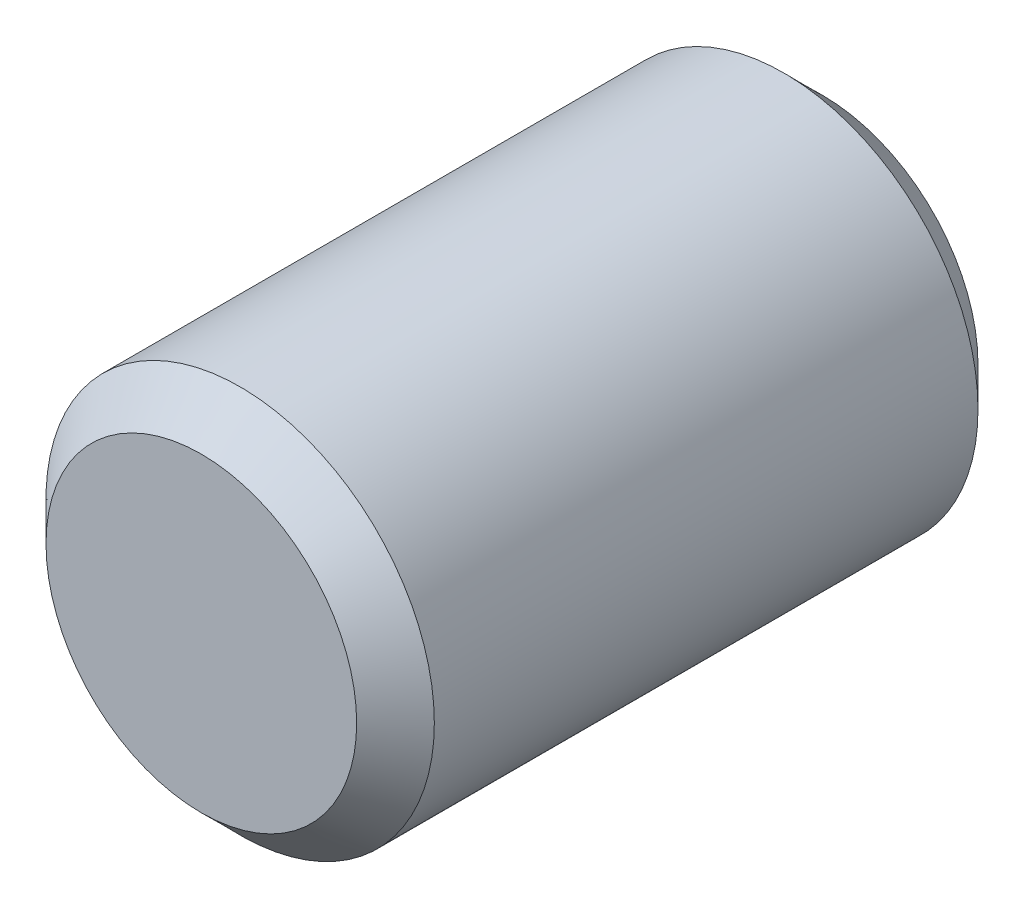
ISO-10303-21;
HEADER;
FILE_DESCRIPTION(('STEP AP214'),'2;1');
FILE_NAME('part.step','',(''),(''),'','','');
FILE_SCHEMA(('AUTOMOTIVE_DESIGN { 1 0 10303 214 1 1 1 1 }'));
ENDSEC;
DATA;
#1=APPLICATION_CONTEXT('core data for automotive mechanical design processes');
#2=APPLICATION_PROTOCOL_DEFINITION('international standard','automotive_design',2000,#1);
#3=PRODUCT_CONTEXT('',#1,'mechanical');
#4=PRODUCT('Part','Part','',(#3));
#5=PRODUCT_RELATED_PRODUCT_CATEGORY('part','',(#4));
#6=PRODUCT_DEFINITION_FORMATION('','',#4);
#7=PRODUCT_DEFINITION_CONTEXT('part definition',#1,'design');
#8=PRODUCT_DEFINITION('design','',#6,#7);
#9=PRODUCT_DEFINITION_SHAPE('','',#8);
#10=(LENGTH_UNIT() NAMED_UNIT(*) SI_UNIT(.MILLI.,.METRE.));
#11=(NAMED_UNIT(*) PLANE_ANGLE_UNIT() SI_UNIT($,.RADIAN.));
#12=(NAMED_UNIT(*) SI_UNIT($,.STERADIAN.) SOLID_ANGLE_UNIT());
#13=UNCERTAINTY_MEASURE_WITH_UNIT(LENGTH_MEASURE(1.E-05),#10,'distance_accuracy_value','');
#14=(GEOMETRIC_REPRESENTATION_CONTEXT(3) GLOBAL_UNCERTAINTY_ASSIGNED_CONTEXT((#13)) GLOBAL_UNIT_ASSIGNED_CONTEXT((#10,
#11,#12)) REPRESENTATION_CONTEXT('',''));
#15=CARTESIAN_POINT('',(0.,0.,0.));
#16=DIRECTION('',(0.,0.,1.));
#17=DIRECTION('',(1.,0.,0.));
#18=AXIS2_PLACEMENT_3D('',#15,#16,#17);
#19=CARTESIAN_POINT('',(0.,0.,8.));
#20=DIRECTION('',(0.,0.,-1.));
#21=DIRECTION('',(-1.,0.,0.));
#22=AXIS2_PLACEMENT_3D('',#19,#20,#21);
#23=CYLINDRICAL_SURFACE('',#22,2.5);
#24=CARTESIAN_POINT('',(0.,0.,0.5));
#25=DIRECTION('',(0.,0.,1.));
#26=DIRECTION('',(1.,0.,0.));
#27=AXIS2_PLACEMENT_3D('',#24,#25,#26);
#28=CIRCLE('',#27,2.5);
#29=CARTESIAN_POINT('',(2.5,0.,0.5));
#30=VERTEX_POINT('',#29);
#31=EDGE_CURVE('E51',#30,#30,#28,.T.);
#32=ORIENTED_EDGE('',*,*,#31,.T.);
#33=EDGE_LOOP('',(#32));
#34=FACE_BOUND('',#33,.T.);
#35=CARTESIAN_POINT('',(0.,0.,7.5));
#36=DIRECTION('',(0.,0.,1.));
#37=DIRECTION('',(1.,0.,0.));
#38=AXIS2_PLACEMENT_3D('',#35,#36,#37);
#39=CIRCLE('',#38,2.5);
#40=CARTESIAN_POINT('',(2.5,0.,7.5));
#41=VERTEX_POINT('',#40);
#42=EDGE_CURVE('E54',#41,#41,#39,.F.);
#43=ORIENTED_EDGE('',*,*,#42,.T.);
#44=EDGE_LOOP('',(#43));
#45=FACE_BOUND('',#44,.T.);
#46=ADVANCED_FACE('F39',(#34,#45),#23,.T.);
#47=CARTESIAN_POINT('',(0.,0.,8.));
#48=DIRECTION('',(0.,0.,1.));
#49=DIRECTION('',(1.,0.,0.));
#50=AXIS2_PLACEMENT_3D('',#47,#48,#49);
#51=PLANE('',#50);
#52=CARTESIAN_POINT('',(0.,0.,8.));
#53=DIRECTION('',(0.,0.,1.));
#54=DIRECTION('',(1.,0.,0.));
#55=AXIS2_PLACEMENT_3D('',#52,#53,#54);
#56=CIRCLE('',#55,2.);
#57=CARTESIAN_POINT('',(2.,0.,8.));
#58=VERTEX_POINT('',#57);
#59=EDGE_CURVE('E10',#58,#58,#56,.T.);
#60=ORIENTED_EDGE('',*,*,#59,.T.);
#61=EDGE_LOOP('',(#60));
#62=FACE_BOUND('',#61,.T.);
#63=ADVANCED_FACE('F72',(#62),#51,.T.);
#64=CARTESIAN_POINT('',(0.,0.,0.));
#65=DIRECTION('',(0.,0.,1.));
#66=DIRECTION('',(1.,0.,0.));
#67=AXIS2_PLACEMENT_3D('',#64,#65,#66);
#68=PLANE('',#67);
#69=CARTESIAN_POINT('',(0.,0.,0.));
#70=DIRECTION('',(0.,0.,1.));
#71=DIRECTION('',(1.,0.,0.));
#72=AXIS2_PLACEMENT_3D('',#69,#70,#71);
#73=CIRCLE('',#72,2.);
#74=CARTESIAN_POINT('',(2.,0.,0.));
#75=VERTEX_POINT('',#74);
#76=EDGE_CURVE('E50',#75,#75,#73,.F.);
#77=ORIENTED_EDGE('',*,*,#76,.T.);
#78=EDGE_LOOP('',(#77));
#79=FACE_BOUND('',#78,.T.);
#80=ADVANCED_FACE('F67',(#79),#68,.F.);
#81=CARTESIAN_POINT('',(0.,0.,0.5));
#82=DIRECTION('',(0.,0.,1.));
#83=DIRECTION('',(1.,0.,0.));
#84=AXIS2_PLACEMENT_3D('',#81,#82,#83);
#85=CONICAL_SURFACE('',#84,2.5,0.78539816339745);
#86=ORIENTED_EDGE('',*,*,#76,.F.);
#87=EDGE_LOOP('',(#86));
#88=FACE_BOUND('',#87,.T.);
#89=ORIENTED_EDGE('',*,*,#31,.F.);
#90=EDGE_LOOP('',(#89));
#91=FACE_BOUND('',#90,.T.);
#92=ADVANCED_FACE('F63',(#88,#91),#85,.T.);
#93=CARTESIAN_POINT('',(0.,0.,8.));
#94=DIRECTION('',(0.,0.,-1.));
#95=DIRECTION('',(-1.,0.,0.));
#96=AXIS2_PLACEMENT_3D('',#93,#94,#95);
#97=CONICAL_SURFACE('',#96,2.,0.785398163397447);
#98=ORIENTED_EDGE('',*,*,#42,.F.);
#99=EDGE_LOOP('',(#98));
#100=FACE_BOUND('',#99,.T.);
#101=ORIENTED_EDGE('',*,*,#59,.F.);
#102=EDGE_LOOP('',(#101));
#103=FACE_BOUND('',#102,.T.);
#104=ADVANCED_FACE('F45',(#100,#103),#97,.T.);
#105=CLOSED_SHELL('',(#46,#63,#80,#92,#104));
#106=MANIFOLD_SOLID_BREP('B2',#105);
#107=ADVANCED_BREP_SHAPE_REPRESENTATION('',(#18,#106),#14);
#108=SHAPE_DEFINITION_REPRESENTATION(#9,#107);
ENDSEC;
END-ISO-10303-21;
